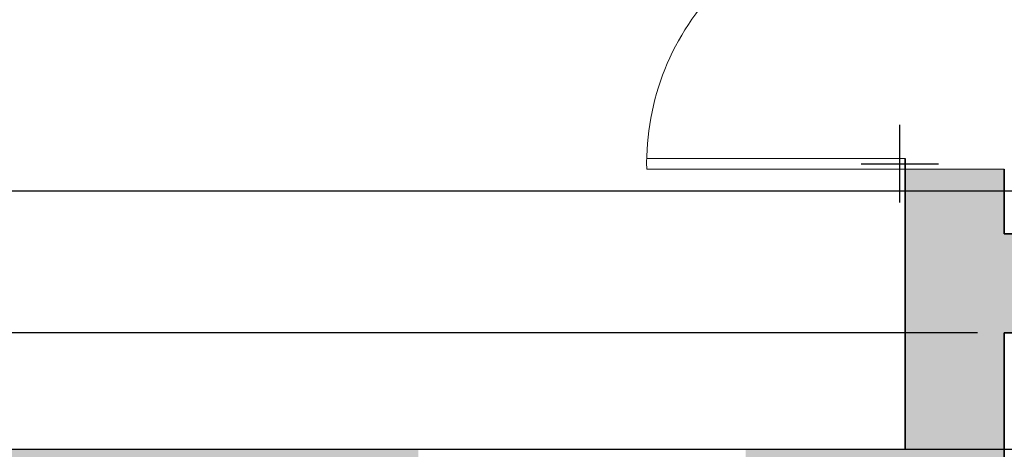
# Model space of a CAD drawing. Units: metres. Extents: x 4298.5 to 4325.2, y 2075 to 2095.8.
# Tile 16 of 35: x 4303.6 to 4305.9, y 2084.8 to 2085.8. Entities that reach past the tile are written whole.
import ezdxf

# ---------------------------------------------------------------- set-up
doc = ezdxf.new("R2010")
doc.units = ezdxf.units.M
for name, color, linetype, lineweight in [('A-ANNO-DIMS', 2, 'Continuous', 18), ('A-DOOR', 3, 'Continuous', 18), ('A-FLOR-CASE', 8, 'Continuous', 18), ('A-WALL', 7, 'Continuous', 35), ('A-WALL-PATT', 252, 'Continuous', 13)]:
    doc.layers.add(name, color=color, linetype=linetype, lineweight=lineweight)
doc.styles.get("Standard").update_dxf_attribs({"font": 'arial.ttf'})
doc.dimstyles.get("Standard").update_dxf_attribs({"dimtxt": 0.18, "dimasz": 0.18, "dimexe": 0.18, "dimexo": 0.0625, "dimgap": 0.09, "dimtad": 0, "dimtih": 1, "dimtoh": 1, "dimdec": 4, "dimzin": 0, "dimdsep": 46, "dimtxsty": 'Standard', "dimcen": 0.09, "dimadec": 0, "dimazin": 0, "dimtfac": 1, "dimtdec": 4, "dimtofl": 0, "dimtmove": 0, "dimatfit": 3, "dimfxl": 1, "dimtolj": 1, "dimtzin": 0, "dimarcsym": 0})

# ---------------------------------------------------------------- blocks, each defined once
blk = doc.blocks.new('DOOR-600-LEAF')
for p, q in [((0, 0), (0, 0.6)), ((0.025, 0), (0.025, 0.6))]:
    blk.add_line(p, q)
blk.add_arc((0.0125, 0.0125), 0.5876, 358.7811, 91.2189)
blk = doc.blocks.new('*D56')
at = {"layer": 'A-ANNO-DIMS', "color": 0, "lineweight": -2, "transparency": 16777216}
for p, q in [((4305.8281, 2085.0581), (4299.0921, 2085.0581)), ((4299.2721, 2084.8781), (4299.2721, 2083.74)), ((4299.2721, 2082.2381), (4299.2721, 2083.3761)), ((4305.8281, 2082.0581), (4299.0921, 2082.0581))]:
    blk.add_line(p, q, dxfattribs=at)
at = {"layer": 'A-ANNO-DIMS', "color": 0, "transparency": 16777216}
for points in [[(4299.2421, 2084.8781), (4299.3021, 2084.8781), (4299.2721, 2085.0581)], [(4299.2421, 2082.2381), (4299.3021, 2082.2381), (4299.2721, 2082.0581)]]:
    blk.add_solid(points, dxfattribs=at)
at = {"layer": 'Defpoints', "color": 0, "transparency": 16777216}
for p in [(4299.2721, 2085.0581), (4305.8906, 2085.0581), (4305.8906, 2082.0581)]:
    blk.add_point(p, dxfattribs=at)
at = {"layer": 'A-ANNO-DIMS', "color": 0, "transparency": 16777216, "insert": (4299.2721, 2083.5581), "char_height": 0.18, "attachment_point": 5}
blk.add_mtext('\\A1;3', dxfattribs=at)
blk = doc.blocks.new('*D58')
at = {"layer": 'A-ANNO-DIMS', "color": 0, "lineweight": -2, "transparency": 16777216}
for p, q in [((4324.5871, 2085.3881), (4324.5871, 2085.5681)), ((4324.5871, 2085.5681), (4324.7671, 2085.5681)), ((4300.7231, 2085.3881), (4324.7671, 2085.3881)), ((4324.5871, 2084.9681), (4324.5871, 2085.2081)), ((4300.7231, 2084.7881), (4324.7671, 2084.7881))]:
    blk.add_line(p, q, dxfattribs=at)
at = {"layer": 'A-ANNO-DIMS', "color": 0, "transparency": 16777216}
for points in [[(4324.5571, 2085.2081), (4324.6171, 2085.2081), (4324.5871, 2085.3881)], [(4324.5571, 2084.9681), (4324.6171, 2084.9681), (4324.5871, 2084.7881)]]:
    blk.add_solid(points, dxfattribs=at)
at = {"layer": 'Defpoints', "color": 0, "transparency": 16777216}
for p in [(4300.6606, 2085.3881), (4324.5871, 2085.3881), (4300.6606, 2084.7881)]:
    blk.add_point(p, dxfattribs=at)
at = {"layer": 'A-ANNO-DIMS', "color": 0, "transparency": 16777216, "insert": (4325.0209, 2085.5681), "char_height": 0.18, "attachment_point": 5}
blk.add_mtext('\\A1;0.6', dxfattribs=at)
blk = doc.blocks.new('*D82')
at = {"layer": 'A-ANNO-DIMS', "color": 0, "lineweight": -2, "transparency": 16777216}
for p, q in [((4304.7983, 2086.1209), (4304.9783, 2086.1209)), ((4304.9783, 2086.1209), (4305.1055, 2085.9936)), ((4305.6481, 2085.3606), (4305.6481, 2085.5406)), ((4305.5581, 2085.4506), (4305.7381, 2085.4506))]:
    blk.add_line(p, q, dxfattribs=at)
at = {"layer": 'A-ANNO-DIMS', "color": 0, "transparency": 16777216}
blk.add_solid([(4305.1267, 2086.0148), (4305.0843, 2085.9724), (4305.2327, 2085.8663)], dxfattribs=at)
at = {"layer": 'Defpoints', "color": 0, "transparency": 16777216}
for p in [(4305.2327, 2085.8663), (4305.6481, 2085.4506)]:
    blk.add_point(p, dxfattribs=at)
at = {"layer": 'A-ANNO-DIMS', "color": 0, "transparency": 16777216, "insert": (4304.1949, 2086.1209), "char_height": 0.18, "attachment_point": 5}
blk.add_mtext('\\A1;3X R0.59', dxfattribs=at)

msp = doc.modelspace()

# ---------------------------------------------------------------- hatches: boundary and pattern name
at = {"layer": 'A-WALL-PATT'}
h = msp.add_hatch(color=256, dxfattribs=at)
h.dxf.hatch_style = 1
h.paths.add_polyline_path([(4308.7606, 2094.4781), (4308.1606, 2094.4781), (4307.4606, 2094.4781), (4307.4606, 2094.2481), (4308.2706, 2094.2481), (4308.2706, 2094.1281), (4308.3906, 2094.1281), (4308.3906, 2094.2481), (4308.7606, 2094.2481)])
h.paths.add_polyline_path([(4310.1206, 2094.4781), (4309.5206, 2094.4781), (4309.5206, 2094.2481), (4309.8906, 2094.2481), (4309.8906, 2092.2481), (4308.3906, 2092.2481), (4308.3906, 2093.4281), (4308.2706, 2093.4281), (4308.2706, 2092.0181), (4309.8906, 2092.0181), (4309.8906, 2087.0181), (4309.7706, 2087.0181), (4309.7706, 2086.7881), (4309.8906, 2086.7881), (4311.9406, 2086.7881), (4311.9406, 2087.0181), (4310.1206, 2087.0181), (4310.1206, 2089.0181), (4310.2406, 2089.0181), (4310.2406, 2089.1381), (4310.1206, 2089.1381), (4310.1206, 2092.0181), (4310.3078, 2092.0181), (4310.3078, 2092.2481), (4310.1206, 2092.2481)])
h.paths.add_polyline_path([(4311.7406, 2092.2481), (4311.0678, 2092.2481), (4311.0678, 2092.0181), (4311.7406, 2092.0181)], flags=17)
h.paths.add_polyline_path([(4313.1733, 2092.2481), (4312.5006, 2092.2481), (4312.5006, 2092.0181), (4313.1733, 2092.0181)])
h.paths.add_polyline_path([(4314.5378, 2092.2481), (4314.1206, 2092.2481), (4313.9333, 2092.2481), (4313.9333, 2092.0181), (4314.1206, 2092.0181), (4314.1206, 2087.0181), (4314.0006, 2087.0181), (4314.0006, 2086.7881), (4314.1206, 2086.7881), (4315.5718, 2086.7881), (4315.5718, 2087.0181), (4314.3506, 2087.0181), (4314.3506, 2092.0181), (4314.5378, 2092.0181)])
h.paths.add_polyline_path([(4315.9706, 2092.2481), (4315.2978, 2092.2481), (4315.2978, 2092.0181), (4315.9706, 2092.0181)])
h.paths.add_polyline_path([(4317.4033, 2092.2481), (4316.7306, 2092.2481), (4316.7306, 2092.0181), (4317.4033, 2092.0181)])
h.paths.add_polyline_path([(4318.9506, 2092.2481), (4318.3506, 2092.2481), (4318.1633, 2092.2481), (4318.1633, 2092.0181), (4318.3506, 2092.0181), (4318.3506, 2091.8981), (4318.5806, 2091.8981), (4318.5806, 2092.0181), (4318.9506, 2092.0181)])
h.paths.add_polyline_path([(4321.0106, 2092.2481), (4319.7106, 2092.2481), (4319.7106, 2092.0181), (4320.0806, 2092.0181), (4320.0806, 2090.0181), (4318.5806, 2090.0181), (4318.5806, 2091.1981), (4318.3506, 2091.1981), (4318.3506, 2090.0181), (4318.3506, 2087.0181), (4318.2306, 2087.0181), (4318.2306, 2086.7881), (4318.3506, 2086.7881), (4318.3506, 2086.3081), (4318.5806, 2086.3081), (4318.5806, 2089.7881), (4321.7806, 2089.7881), (4321.7806, 2090.0181), (4320.2006, 2090.0181), (4320.2006, 2092.0181), (4321.0106, 2092.0181)])
h.paths.add_polyline_path([(4322.8106, 2092.2481), (4321.7706, 2092.2481), (4321.7706, 2092.0181), (4322.5806, 2092.0181), (4322.5806, 2091.2831), (4322.8106, 2091.2831)])
h.paths.add_polyline_path([(4322.8106, 2090.5231), (4322.5806, 2090.5231), (4322.5806, 2089.7881), (4322.5806, 2089.5254), (4322.8106, 2089.5254), (4322.8106, 2090.0181)])
h.paths.add_polyline_path([(4322.8106, 2088.7654), (4322.5806, 2088.7654), (4322.5806, 2087.6681), (4322.8106, 2087.6681)])
h.paths.add_polyline_path([(4322.8106, 2086.9081), (4322.5806, 2086.9081), (4322.5806, 2085.8107), (4322.8106, 2085.8107)])
h.paths.add_polyline_path([(4322.8106, 2085.0507), (4322.5806, 2085.0507), (4322.5806, 2084.7881), (4318.5806, 2084.7881), (4318.5806, 2085.0581), (4318.5806, 2085.4081), (4318.3506, 2085.4081), (4318.3506, 2084.5581), (4318.3506, 2080.8581), (4318.4706, 2080.8581), (4318.4706, 2082.3281), (4319.2606, 2082.3281), (4319.2606, 2082.5581), (4318.5806, 2082.5581), (4318.5806, 2084.5581), (4320.0806, 2084.5581), (4320.0806, 2083.9381), (4320.3106, 2083.9381), (4320.3106, 2084.5581), (4322.8106, 2084.5581)])
h.paths.add_polyline_path([(4320.3106, 2083.1781), (4320.0806, 2083.1781), (4320.0806, 2082.5581), (4319.9606, 2082.5581), (4319.9606, 2082.3281), (4320.0806, 2082.3281), (4320.0806, 2081.5731), (4320.3106, 2081.5731)], flags=17)
h.paths.add_polyline_path([(4320.3106, 2080.8131), (4320.0806, 2080.8131), (4320.0806, 2080.0581), (4318.4286, 2080.0581), (4318.4286, 2079.8281), (4320.3106, 2079.8281)])
h.paths.add_polyline_path([(4317.3506, 2085.2881), (4316.5718, 2085.2881), (4316.5718, 2085.0581), (4317.3506, 2085.0581)])
h.paths.add_polyline_path([(4315.5718, 2085.2881), (4314.8434, 2085.2881), (4314.8434, 2085.0581), (4315.5718, 2085.0581)])
h.paths.add_polyline_path([(4313.8434, 2085.2881), (4312.9406, 2085.2881), (4312.9406, 2085.0581), (4313.8434, 2085.0581)])
h.paths.add_polyline_path([(4311.9406, 2085.2881), (4311.4406, 2085.2881), (4311.4406, 2085.0581), (4311.9406, 2085.0581)])
h.paths.add_polyline_path([(4317.3306, 2087.0181), (4316.5718, 2087.0181), (4316.5718, 2086.7881), (4317.3306, 2086.7881)])
h.paths.add_polyline_path([(4313.1006, 2089.1381), (4311.1406, 2089.1381), (4311.1406, 2089.0181), (4312.9806, 2089.0181), (4312.9806, 2087.0181), (4312.9406, 2087.0181), (4312.9406, 2086.7881), (4313.1006, 2086.7881), (4313.1006, 2087.0181)])
h.paths.add_polyline_path([(4307.5515, 2087.0181), (4305.8906, 2087.0181), (4305.8906, 2092.2481), (4305.8906, 2094.2481), (4306.7006, 2094.2481), (4306.7006, 2094.4781), (4305.6606, 2094.4781), (4305.6606, 2092.2481), (4305.2906, 2092.2481), (4305.2906, 2092.0181), (4305.6606, 2092.0181), (4305.6606, 2090.0181), (4304.1606, 2090.0181), (4304.1606, 2091.1981), (4304.0406, 2091.1981), (4304.0406, 2089.9081), (4301.5606, 2089.9081), (4301.5606, 2089.7881), (4304.0406, 2089.7881), (4305.6606, 2089.7881), (4305.6606, 2086.6381), (4305.8906, 2086.6381), (4305.8906, 2086.7881), (4307.5515, 2086.7881)])
h.paths.add_polyline_path([(4307.5515, 2085.2881), (4305.8906, 2085.2881), (4305.8906, 2085.4381), (4305.6606, 2085.4381), (4305.6606, 2084.7881), (4305.2906, 2084.7881), (4305.2906, 2084.5581), (4305.6606, 2084.5581), (4305.6606, 2084.02), (4305.8906, 2084.02), (4305.8906, 2084.5581), (4305.8906, 2085.0581), (4307.5515, 2085.0581)])
h.paths.add_polyline_path([(4310.2406, 2085.2881), (4308.5515, 2085.2881), (4308.5515, 2085.0581), (4310.2406, 2085.0581)])
h.paths.add_polyline_path([(4317.4286, 2080.0581), (4316.5718, 2080.0581), (4316.5718, 2079.8281), (4317.4286, 2079.8281)])
h.paths.add_polyline_path([(4315.5718, 2080.0581), (4314.8434, 2080.0581), (4314.8434, 2079.8281), (4315.5718, 2079.8281)])
h.paths.add_polyline_path([(4313.8434, 2080.0581), (4312.9406, 2080.0581), (4312.9406, 2079.8281), (4313.8434, 2079.8281)])
h.paths.add_polyline_path([(4311.9406, 2080.0581), (4311.4406, 2080.0581), (4311.4406, 2079.8281), (4311.9406, 2079.8281)])
h.paths.add_polyline_path([(4310.2406, 2080.0581), (4310.1206, 2080.0581), (4310.1206, 2084.0381), (4309.8906, 2084.0381), (4309.8906, 2080.0581), (4309.1606, 2080.0581), (4309.1606, 2079.8281), (4310.2406, 2079.8281)])
h.paths.add_polyline_path([(4308.1606, 2080.0581), (4307.5106, 2080.0581), (4307.5106, 2080.1781), (4307.3906, 2080.1781), (4307.3906, 2080.0581), (4305.8906, 2080.0581), (4305.8906, 2080.567), (4305.6606, 2080.567), (4305.6606, 2079.8281), (4308.1606, 2079.8281)])
h.paths.add_polyline_path([(4307.5106, 2081.9381), (4309.0906, 2081.9381), (4309.0906, 2082.0581), (4305.8906, 2082.0581), (4305.8906, 2083.26), (4305.6606, 2083.26), (4305.6606, 2081.327), (4305.8906, 2081.327), (4305.8906, 2081.9381), (4307.3906, 2081.9381), (4307.3906, 2080.8781), (4307.5106, 2080.8781)])
h.paths.add_polyline_path([(4304.5306, 2084.7881), (4302.7306, 2084.7881), (4302.7306, 2084.5581), (4304.5306, 2084.5581)])
h.paths.add_polyline_path([(4301.9706, 2084.7881), (4300.6606, 2084.7881), (4300.6606, 2085.0249), (4300.4306, 2085.0249), (4300.4306, 2084.5581), (4301.9706, 2084.5581)])
h.paths.add_polyline_path([(4300.6606, 2086.8843), (4300.4306, 2086.8843), (4300.4306, 2085.7849), (4300.6606, 2085.7849)])
h.paths.add_polyline_path([(4300.6606, 2089.1618), (4300.4306, 2089.1618), (4300.4306, 2087.6443), (4300.6606, 2087.6443)])
h.paths.add_polyline_path([(4300.6606, 2091.0212), (4300.4306, 2091.0212), (4300.4306, 2089.9218), (4300.6606, 2089.9218)])
h.paths.add_polyline_path([(4300.6606, 2092.0181), (4301.9706, 2092.0181), (4301.9706, 2092.2481), (4300.4306, 2092.2481), (4300.4306, 2091.7812), (4300.6606, 2091.7812)])
h.paths.add_polyline_path([(4304.5306, 2092.2481), (4302.7306, 2092.2481), (4302.7306, 2092.0181), (4304.0406, 2092.0181), (4304.0406, 2091.8981), (4304.1606, 2091.8981), (4304.1606, 2092.0181), (4304.5306, 2092.0181)], flags=17)

# ---------------------------------------------------------------- linework, layer by layer
at = {"layer": 'A-DOOR'}
msp.add_line((4305.8906, 2085.4381), (4305.6606, 2085.4381), dxfattribs=at)
at = {"layer": 'A-FLOR-CASE'}
msp.add_line((4305.6606, 2085.3881), (4300.6606, 2085.3881), dxfattribs=at)
at = {"layer": 'A-WALL'}
for p, q in [((4305.6606, 2085.4631), (4305.6606, 2084.7881)), ((4305.8906, 2085.4381), (4305.8906, 2085.2881)), ((4305.8906, 2085.2881), (4310.2406, 2085.2881)), ((4305.8906, 2085.0581), (4310.2406, 2085.0581)), ((4305.8906, 2085.0581), (4305.8906, 2084.5581))]:
    msp.add_line(p, q, dxfattribs=at)

# ---------------------------------------------------------------- block references
at = {"layer": 'A-DOOR', "rotation": 89.9999999966095}
msp.add_blockref('DOOR-600-LEAF', (4305.6606, 2085.4381), dxfattribs=at)

# ---------------------------------------------------------------- dimensions: what is measured, and where the dimension line sits
at = {"layer": 'A-ANNO-DIMS'}
dim = msp.add_radius_dim(center=(4305.6481, 2085.4506), mpoint=(4305.2327, 2085.8663), text='3X <>', dimstyle='Standard', override={"dimdec": 2, "dimlfac": 1, "dimrnd": 0, "dimzin": 0, "dimdsep": 46, "dimlunit": 2}, dxfattribs=at)
dim.commit()
dim.dimension.update_dxf_attribs({"geometry": '*D82', "text_midpoint": (4304.1949, 2086.1209)})
for base, p1, p2, override, picture, middle in [((4324.5871, 2085.3881), (4300.6606, 2084.7881), (4300.6606, 2085.3881), {"dimdec": 1, "dimlfac": 1, "dimrnd": 0, "dimzin": 0, "dimdsep": 46, "dimlunit": 2}, '*D58', (4325.0209, 2085.5681)), ((4299.2721, 2085.0581), (4305.8906, 2082.0581), (4305.8906, 2085.0581), {"dimdec": 0, "dimlfac": 1, "dimrnd": 0, "dimzin": 0, "dimdsep": 46, "dimlunit": 2}, '*D56', (4299.2721, 2083.5581))]:
    dim = msp.add_linear_dim(base=base, p1=p1, p2=p2, angle=90, dimstyle='Standard', override=override, dxfattribs=at)
    dim.commit()
    dim.dimension.update_dxf_attribs({"geometry": picture, "text_midpoint": middle})

doc.saveas('drawing.dxf')
